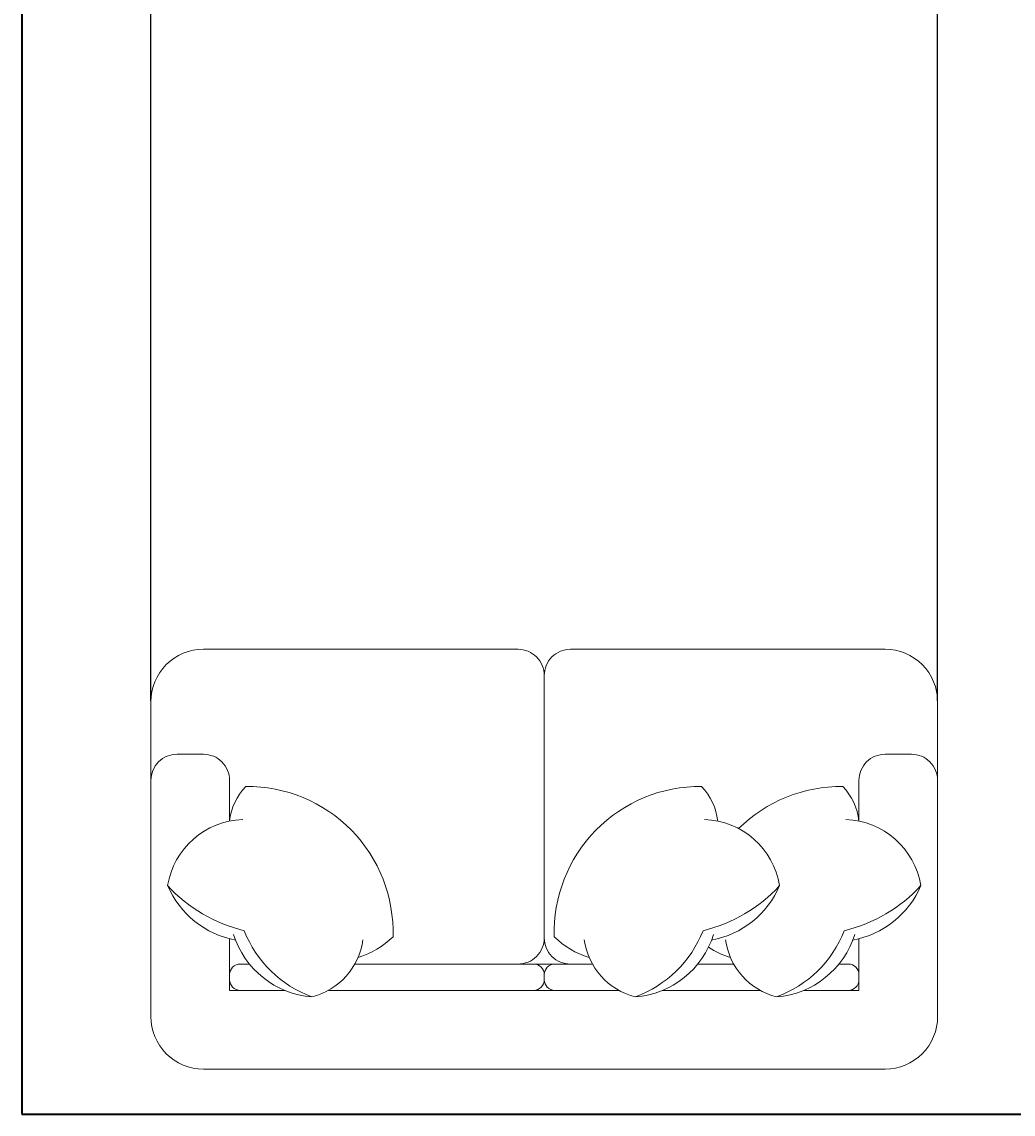
# Model space of a CAD drawing. Units: inches. Extents: x 1088 to 1703, y 668 to 1875.
# Tile 9 of 45: x 1175 to 1244, y 1419 to 1496. Entities that reach past the tile are written whole.
import ezdxf

# ---------------------------------------------------------------- set-up
doc = ezdxf.new("R2010")
doc.units = ezdxf.units.IN
for name, color, linetype, lineweight in [('A-ANNO-DIMS', 2, 'Continuous', 18), ('A-FURN', 8, 'Continuous', 13), ('A-WALL', 7, 'Continuous', 35)]:
    doc.layers.add(name, color=color, linetype=linetype, lineweight=lineweight)
doc.styles.get("Standard").update_dxf_attribs({"font": 'arial.ttf'})
doc.dimstyles.get("Standard").update_dxf_attribs({"dimtxt": 0.18, "dimasz": 0.18, "dimexe": 0.18, "dimexo": 0.0625, "dimgap": 0.09, "dimtad": 0, "dimtih": 1, "dimtoh": 1, "dimdec": 4, "dimzin": 0, "dimdsep": 46, "dimtxsty": 'Standard', "dimcen": 0.09, "dimadec": 0, "dimazin": 0, "dimtfac": 1, "dimtdec": 4, "dimtofl": 0, "dimtmove": 0, "dimatfit": 3, "dimfxl": 1, "dimtolj": 1, "dimtzin": 0, "dimarcsym": 0})

# ---------------------------------------------------------------- blocks, each defined once
blk = doc.blocks.new('*D35')
at = {"layer": 'A-ANNO-DIMS', "color": 0, "lineweight": -2, "transparency": 16777216}
for p, q in [((1183.893, 1448.103), (1183.893, 1857.788)), ((1184.073, 1857.608), (1211.072, 1857.608)), ((1238.859, 1857.608), (1211.86, 1857.608)), ((1239.039, 1448.103), (1239.039, 1857.788))]:
    blk.add_line(p, q, dxfattribs=at)
at = {"layer": 'A-ANNO-DIMS', "color": 0, "transparency": 16777216}
for points in [[(1184.073, 1857.638), (1184.073, 1857.578), (1183.893, 1857.608)], [(1238.859, 1857.638), (1238.859, 1857.578), (1239.039, 1857.608)]]:
    blk.add_solid(points, dxfattribs=at)
at = {"layer": 'Defpoints', "color": 0, "transparency": 16777216}
for p in [(1239.039, 1857.608), (1183.893, 1448.04), (1239.039, 1448.04)]:
    blk.add_point(p, dxfattribs=at)
at = {"layer": 'A-ANNO-DIMS', "color": 0, "transparency": 16777216, "insert": (1211.466, 1857.608), "char_height": 0.18, "attachment_point": 5}
blk.add_mtext('\\A1;55.15', dxfattribs=at)

msp = doc.modelspace()

# ---------------------------------------------------------------- linework, layer by layer
at = {"layer": 'A-FURN', "ltscale": 0.03}
msp.add_lwpolyline([(1209.628, 1451.717, -0.414214), (1211.466, 1449.878, -0.414214), (1213.304, 1451.717), (1235.363, 1451.717, -0.414214), (1239.039, 1448.04), (1239.039, 1425.982, -0.414214), (1235.363, 1422.305), (1187.569, 1422.305, -0.414214), (1183.893, 1425.982), (1183.893, 1448.04, -0.414214), (1187.569, 1451.717), (1209.628, 1451.717, -0.414214), (1211.466, 1449.878, -0.414214), (1213.304, 1451.717)], format="xyb", dxfattribs=at)
at = {"layer": 'A-FURN'}
for points in [[(1209.628, 1429.658, 0.414214), (1211.466, 1431.496), (1211.466, 1449.878, 0.414214)], [(1213.304, 1429.658, -0.414214), (1211.466, 1431.496), (1211.466, 1449.878, -0.414214)], [(1183.893, 1442.526, -0.414214), (1185.731, 1444.364), (1187.569, 1444.364, -0.414214), (1189.408, 1442.526), (1189.408, 1439.678)], [(1233.525, 1439.678), (1233.525, 1442.526, -0.414214), (1235.363, 1444.364), (1237.201, 1444.364, -0.414214), (1239.039, 1442.526)], [(1189.404, 1439.677, -0.165541), (1190.541, 1442.106, -0.425989), (1200.864, 1431.575, -0.121523), (1198.414, 1430.124, 7.115464)], [(1223.626, 1439.677, 0.165541), (1222.489, 1442.106, 0.425989), (1212.165, 1431.575, 0.121523), (1214.616, 1430.124, -7.115464)], [(1233.529, 1439.677, 0.165541), (1232.391, 1442.106, 0.200231), (1225.094, 1439.148, 0.121523)], [(1190.33, 1439.789, 0.356772), (1185.063, 1435.155, 0.249542), (1189.835, 1431.337, -9.61688)], [(1222.7, 1439.789, -0.356772), (1227.967, 1435.155, -0.249542), (1223.194, 1431.337, 9.61688)], [(1232.602, 1439.789, -0.356772), (1237.869, 1435.155, -0.249542), (1233.097, 1431.337, 9.61688)], [(1185.063, 1435.155, 0.14773), (1190.435, 1431.996, 0.213343), (1195.176, 1427.363, 0.178662)], [(1227.967, 1435.155, -0.14773), (1222.594, 1431.996, -0.213343), (1217.854, 1427.363, -0.178662)], [(1237.869, 1435.155, -0.14773), (1232.497, 1431.996, -0.213343), (1227.756, 1427.363, -0.178662)], [(1189.693, 1431.744, 0.306663), (1195.176, 1427.363, 0.30633), (1198.758, 1431.364, -0.872847)], [(1209.628, 1429.658, 0.414214), (1211.466, 1431.496)], [(1213.304, 1429.658, -0.414214), (1211.466, 1431.496)], [(1223.337, 1431.744, -0.306663), (1217.854, 1427.363, -0.30633), (1214.272, 1431.364, 0.872847)], [(1233.239, 1431.744, -0.306663), (1227.756, 1427.363, -0.30633), (1224.175, 1431.364, 0.872847)], [(1229.657, 1427.82), (1233.525, 1427.82), (1233.525, 1431.432, -0.414214)], [(1222.977, 1430.842, 0.071865), (1224.518, 1430.124, -7.115464)], [(1190.81, 1429.658), (1190.143, 1429.658, 0.414214), (1189.408, 1428.923), (1189.408, 1428.555, 0.414214), (1190.143, 1427.82)], [(1196.333, 1427.82), (1210.731, 1427.82, 0.414214), (1211.466, 1428.555), (1211.466, 1428.923, 0.414214), (1210.731, 1429.658), (1198.184, 1429.658, 0.414214)], [(1216.697, 1427.82), (1212.201, 1427.82, -0.414214), (1211.466, 1428.555), (1211.466, 1428.923, -0.414214), (1212.201, 1429.658), (1214.846, 1429.658, -0.414214)], [(1222.219, 1429.658), (1224.748, 1429.658, -0.414214)], [(1232.122, 1429.658), (1232.789, 1429.658, -0.414214), (1233.525, 1428.923), (1233.525, 1428.555, -0.414214), (1232.789, 1427.82)], [(1190.143, 1427.82), (1193.275, 1427.82, 0.414214)], [(1226.599, 1427.82), (1219.755, 1427.82, -0.414214)], [(1232.789, 1427.82), (1229.657, 1427.82, -0.414214)]]:
    msp.add_lwpolyline(points, format="xyb", dxfattribs=at)
for points in [[(1189.408, 1431.432), (1189.408, 1427.82), (1193.275, 1427.82)], [(1196.333, 1427.82), (1216.697, 1427.82)], [(1219.755, 1427.82), (1226.599, 1427.82)]]:
    msp.add_lwpolyline(points, dxfattribs=at)
msp.add_lwpolyline([(1210.731, 1427.82), (1212.201, 1427.82, -0.414214), (1211.466, 1428.555), (1211.466, 1428.923, -0.414214), (1212.201, 1429.658), (1210.731, 1429.658, -0.414214), (1211.466, 1428.923), (1211.466, 1428.555, -0.414214)], format="xyb", close=True, dxfattribs=at)
at = {"layer": 'A-WALL'}
for p, q in [((1174.845, 1644.558), (1174.845, 1419.144)), ((1174.845, 1419.144), (1310.352, 1419.144))]:
    msp.add_line(p, q, dxfattribs=at)

# ---------------------------------------------------------------- dimensions: what is measured, and where the dimension line sits
at = {"layer": 'A-ANNO-DIMS'}
dim = msp.add_linear_dim(base=(1239.039, 1857.608), p1=(1183.893, 1448.04), p2=(1239.039, 1448.04), dimstyle='Standard', override={"dimdec": 2, "dimlfac": 1, "dimrnd": 0, "dimzin": 0, "dimdsep": 46, "dimlunit": 2}, dxfattribs=at)
dim.commit()
dim.dimension.update_dxf_attribs({"geometry": '*D35', "text_midpoint": (1211.466, 1857.608)})

doc.saveas('drawing.dxf')
